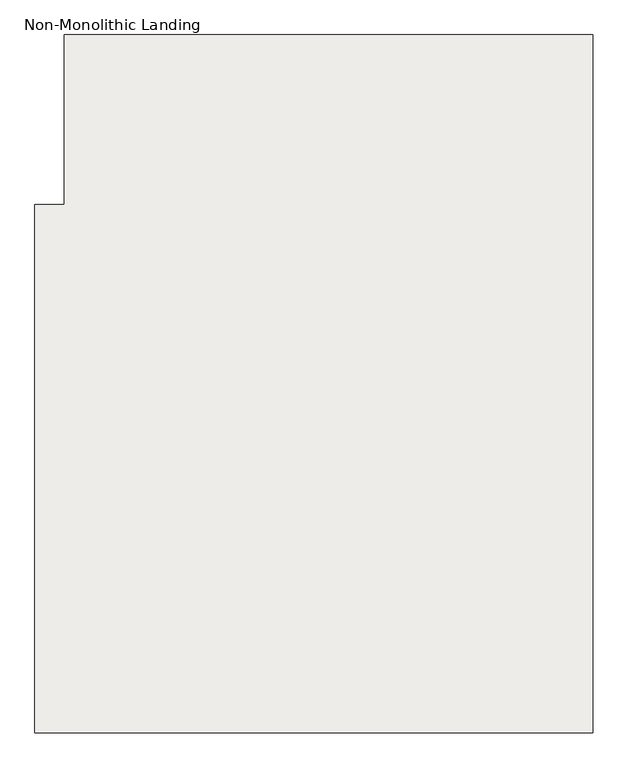
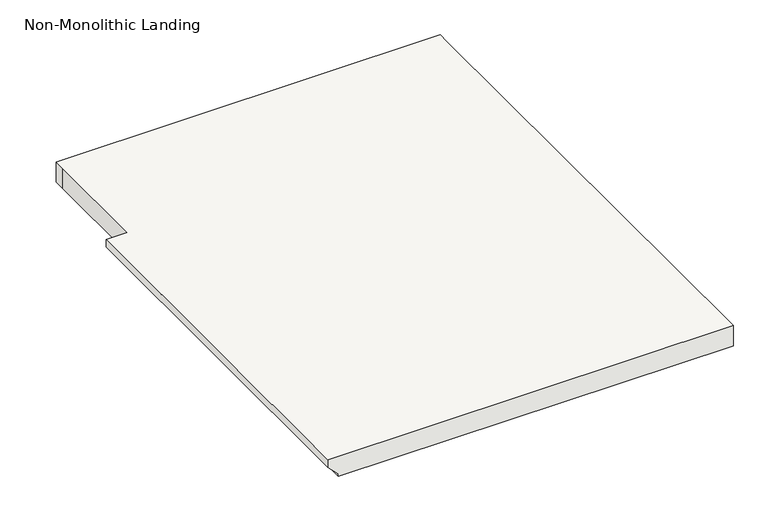
"""IFC4 building model written with IfcOpenShell, lengths in millimetres: slab geometry, Non-Monolithic Landing."""

from ifc_helpers import new_model, si_unit, origin, place, context, project, spatial, faceted_brep, source, transform, mapped, element, save


def non_monolithic_landing_4baf8b2c(model_context):
    return source(origin(), model_context, "Body", "Brep", [
        faceted_brep([(8906.0423568, -10720.6073314, 4392.5289474), (8906.0423568, -10720.6073314, 4411.5789474), (8906.0423568, -9806.2073314, 4411.5789474), (8906.0423568, -9806.2073314, 4392.5289474), (8931.4423568, -10720.6073314, 4367.1289474), (8931.4423568, -9806.2073314, 4367.1289474), (9871.2423568, -10720.6073314, 4411.5789474), (9871.2423568, -9537.7746824, 4411.5789474), (9871.2423568, -9512.3746824, 4411.5789474), (8956.8423568, -9512.3746824, 4411.5789474), (8956.8423568, -9537.7746824, 4411.5789474), (8956.8423568, -9806.2073314, 4411.5789474), (8931.4423568, -10720.6073314, 4360.7789474), (8931.4423568, -9806.2073314, 4360.7789474), (8956.8423568, -9806.2073314, 4360.7789474), (8956.8423568, -9537.7746824, 4360.7789474), (8956.8423568, -9512.3746824, 4360.7789474), (9871.2423568, -9512.3746824, 4360.7789474), (9871.2423568, -9537.7746824, 4360.7789474), (9871.2423568, -10720.6073314, 4360.7789474)], [[[0, 1, 2, 3]], [[4, 0, 3, 5]], [[6, 7, 8, 9, 10, 11, 2, 1]], [[12, 13, 14, 15, 16, 17, 18, 19]], [[13, 12, 4, 5]], [[6, 1, 0, 4, 12, 19]], [[7, 6, 19, 18]], [[8, 7, 18, 17]], [[9, 8, 17, 16]], [[10, 9, 16, 15]], [[11, 10, 15, 14]], [[2, 11, 14, 13, 5, 3]]]),
    ])


if __name__ == "__main__":
    model = new_model("IFC4")
    model_context = context("Model", 3, world=origin())
    ifc_project = project(units=[si_unit("LENGTHUNIT", "METRE", prefix="MILLI")], contexts=[model_context])
    site = spatial("IfcSite", under=ifc_project)
    building = spatial("IfcBuilding", under=site)
    placement = place(None, origin())
    non_monolithic_landing_shape = non_monolithic_landing_4baf8b2c(model_context)
    element("IfcSlab", 1, ObjectType="Non-Monolithic Landing", at=placement, inside=building, context=model_context, shape_type="MappedRepresentation", body=[
        mapped(non_monolithic_landing_shape, transform((0.0, 0.0, 0.0), x_axis=(1.0, 0.0, 0.0), y_axis=(0.0, 1.0, 0.0), z_axis=(0.0, 0.0, 1.0))),
    ])
    save(model, "model.ifc")

# Revit data of these elements
# Element 1 (IfcSlab, "Non-Monolithic Landing")
#   Materials on its faces: "MARBLE STAIRS 6\""
# Materials
#   "MARBLE STAIRS 6\"": class "Generic", colour RGB 120 120 120, transparency 0, Cost = 0
